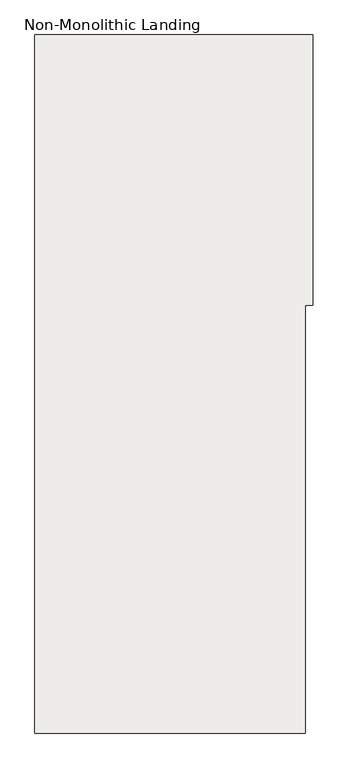
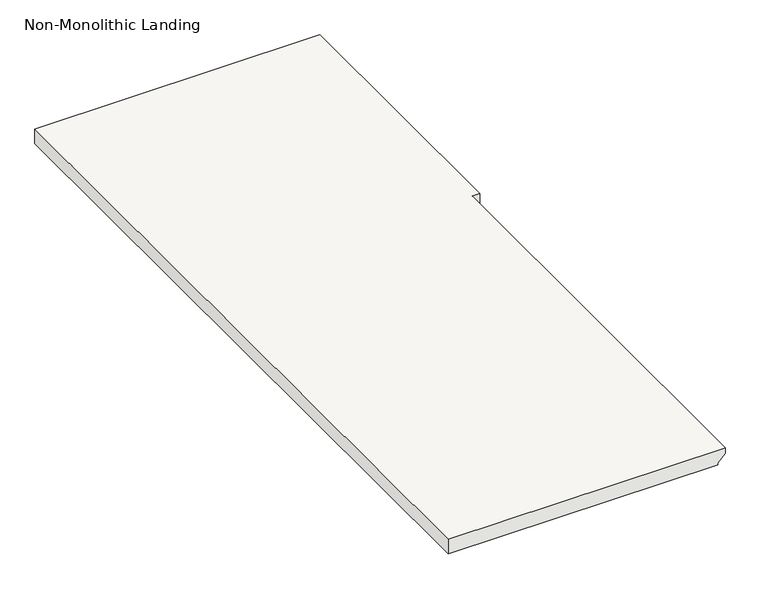
"""IFC4 building model written with IfcOpenShell, lengths in millimetres: slab geometry, Non-Monolithic Landing."""

from ifc_helpers import new_model, si_unit, origin, place, context, project, spatial, faceted_brep, source, transform, mapped, element, save


def non_monolithic_landing_094f5741(model_context):
    return source(origin(), model_context, "Body", "Brep", [
        faceted_brep([(20207.1136801, 4166.5752787, 5746.75), (20181.7136801, 4166.5752787, 5721.35), (20181.7136801, 5080.9752787, 5721.35), (20207.1136801, 5080.9752787, 5746.75), (20207.1136801, 5614.3752787, 5765.8), (20232.5136801, 5614.3752787, 5765.8), (20232.5136801, 6528.7752787, 5765.8), (20207.1136801, 6528.7752787, 5765.8), (19292.7136801, 6528.7752787, 5765.8), (19292.7136801, 4166.5752787, 5765.8), (20207.1136801, 4166.5752787, 5765.8), (20181.7136801, 5080.9752787, 5715.0), (20181.7136801, 4166.5752787, 5715.0), (19292.7136801, 4166.5752787, 5715.0), (19292.7136801, 6528.7752787, 5715.0), (20207.1136801, 6528.7752787, 5715.0), (20232.5136801, 6528.7752787, 5715.0), (20232.5136801, 5614.3752787, 5715.0), (20207.1136801, 5614.3752787, 5715.0), (20207.1136801, 5080.9752787, 5715.0)], [[[0, 1, 2, 3]], [[4, 5, 6, 7, 8, 9, 10]], [[11, 12, 13, 14, 15, 16, 17, 18, 19]], [[12, 11, 2, 1]], [[11, 19, 3, 2]], [[4, 10, 0, 3, 19, 18]], [[5, 4, 18, 17]], [[6, 5, 17, 16]], [[7, 6, 16, 15]], [[8, 7, 15, 14]], [[9, 8, 14, 13]], [[10, 9, 13, 12, 1, 0]]]),
    ])


if __name__ == "__main__":
    model = new_model("IFC4")
    model_context = context("Model", 3, world=origin())
    ifc_project = project(units=[si_unit("LENGTHUNIT", "METRE", prefix="MILLI")], contexts=[model_context])
    site = spatial("IfcSite", under=ifc_project)
    building = spatial("IfcBuilding", under=site)
    placement = place(None, origin())
    non_monolithic_landing_shape = non_monolithic_landing_094f5741(model_context)
    element("IfcSlab", 1, ObjectType="Non-Monolithic Landing", at=placement, inside=building, context=model_context, shape_type="MappedRepresentation", body=[
        mapped(non_monolithic_landing_shape, transform((0.0, 0.0, 0.0), x_axis=(1.0, 0.0, 0.0), y_axis=(0.0, 1.0, 0.0), z_axis=(0.0, 0.0, 1.0))),
    ])
    save(model, "model.ifc")
